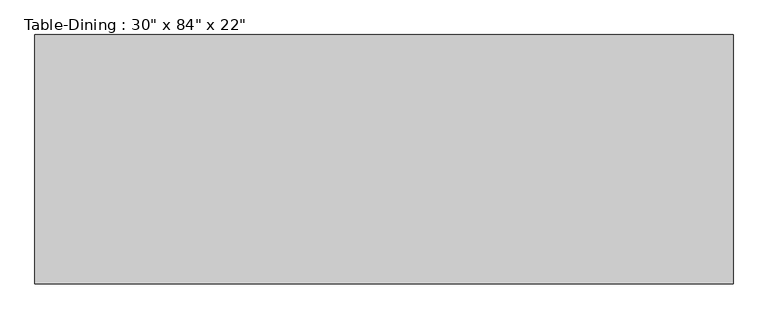
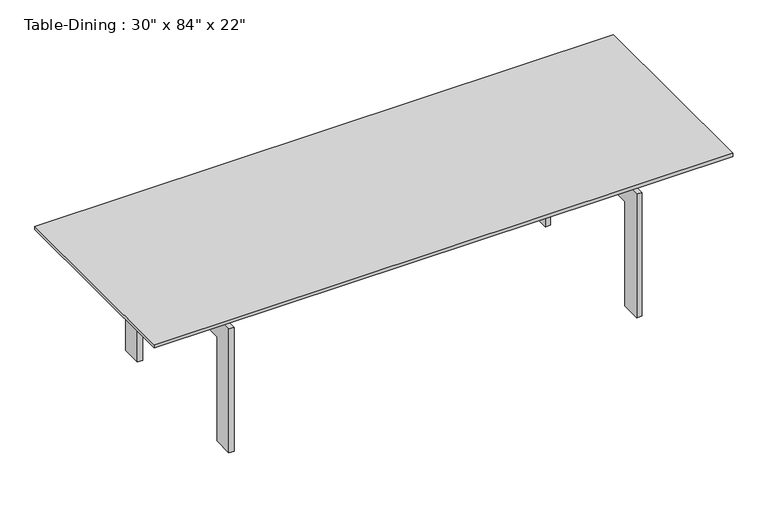
"""IFC4 building model written with IfcOpenShell, lengths in millimetres: furniture geometry."""

from ifc_helpers import new_model, si_unit, frame, origin, place, context, project, spatial, polyline, outline, extrude, source, transform, mapped, element, save


def furniture_92191dda(model_context):
    return source(origin(), model_context, "Body", "SweptSolid", [
        extrude(outline(polyline([(983.4657667, 297.7823857), (983.4657667, 272.3823857), (-946.9342333, 272.3823857), (-946.9342333, 297.7823857), (983.4657667, 297.7823857)])), frame((0.0, 0.0, 482.6), z_axis=(0.0, 0.0, 1.0), x_axis=(1.0, 0.0, 0.0)), (0.0, 0.0, 1.0), 63.5),
        extrude(outline(polyline([(983.4657667, -82.5889222), (983.4657667, -107.9889222), (-946.9342333, -107.9889222), (-946.9342333, -82.5889222), (983.4657667, -82.5889222)])), frame((0.0, 0.0, 482.6), z_axis=(0.0, 0.0, 1.0), x_axis=(1.0, 0.0, 0.0)), (0.0, 0.0, 1.0), 63.5),
        extrude(outline(polyline([(425.4110778, 0.0), (349.2110778, 0.0), (349.2110778, 406.4), (-158.7889222, 406.4), (-158.7889222, 0.0), (-234.9889222, 0.0), (-234.9889222, 482.6), (425.4110778, 482.6), (425.4110778, 0.0)])), frame((761.2157667, 0.0, 0.0), z_axis=(1.0, 0.0, 0.0), x_axis=(0.0, 1.0, 0.0)), (0.0, 0.0, 1.0), 19.05),
        extrude(outline(polyline([(425.4110778, 482.6), (425.4110778, 0.0), (349.2110778, 0.0), (349.2110778, 406.4), (-158.7889222, 406.4), (-158.7889222, 0.0), (-234.9889222, 0.0), (-234.9889222, 482.6), (425.4110778, 482.6)])), frame((-743.7342333, 0.0, 0.0), z_axis=(1.0, 0.0, 0.0), x_axis=(0.0, 1.0, 0.0)), (0.0, 0.0, 1.0), 19.05),
        extrude(outline(polyline([(1085.0657667, 476.2110778), (1085.0657667, -285.7889222), (-1048.5342333, -285.7889222), (-1048.5342333, 476.2110778), (1085.0657667, 476.2110778)])), frame((0.0, 0.0, 546.1), z_axis=(0.0, 0.0, 1.0), x_axis=(1.0, 0.0, 0.0)), (0.0, 0.0, 1.0), 12.7),
    ])


if __name__ == "__main__":
    model = new_model("IFC4")
    model_context = context("Model", 3, world=origin())
    ifc_project = project(units=[si_unit("LENGTHUNIT", "METRE", prefix="MILLI")], contexts=[model_context])
    site = spatial("IfcSite", under=ifc_project)
    building = spatial("IfcBuilding", under=site)
    placement = place(None, origin())
    furniture_shape = furniture_92191dda(model_context)
    element("IfcFurniture", 1, ObjectType="Table-Dining : 30\" x 84\" x 22\"", at=placement, inside=building, context=model_context, shape_type="MappedRepresentation", body=[
        mapped(furniture_shape, transform((0.0, 0.0, 0.0), x_axis=(1.0, 0.0, 0.0), y_axis=(0.0, 1.0, 0.0), z_axis=(0.0, 0.0, 1.0))),
    ])
    save(model, "model.ifc")

# Revit data of these elements
# Type "Table-Dining : 30\" x 84\" x 22\""
#   Assembly Code = "E2020200"
#   Height = 1' - 10"
#   Length = 7' - 0"
#   Width = 2' - 6"
#   Base Material = Steel, Chrome Plated
#   Top Material = Glass - Clear, Grey
#   Default Elevation = 0
# Element 1 (IfcFurniture, "Table-Dining : 30\" x 84\" x 22\"")
#   Materials on its faces: "Steel, Chrome Plated", "Glass - Clear, Grey"
# Materials
#   "Steel, Chrome Plated": class "Metal", colour RGB 17 17 17, transparency 0, Description = "Chromiuim plated steel", Cost = 0
#   "Glass - Clear, Grey": class "Glass", colour RGB 252 255 255, transparency 0.64
